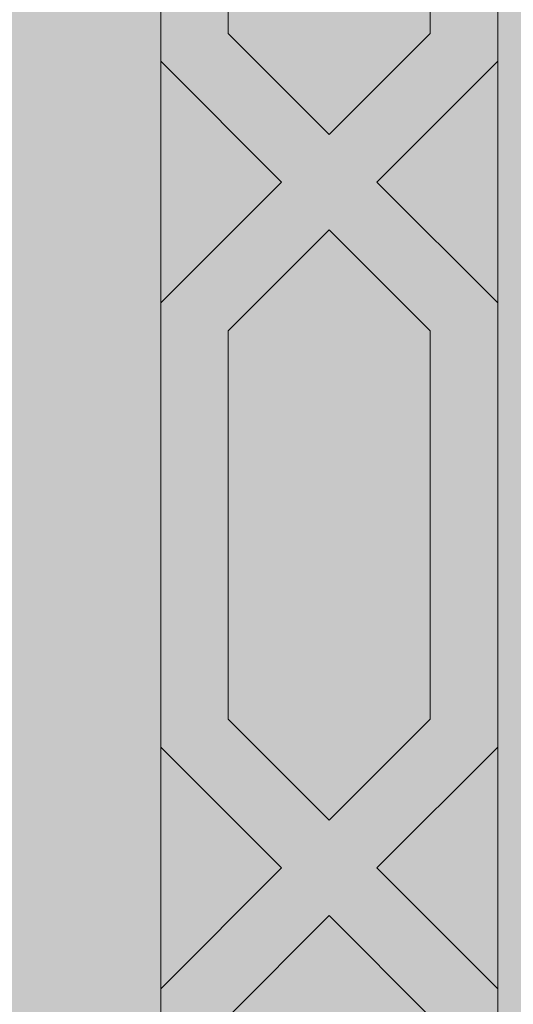
# Model space of a CAD drawing. Units: inches. Extents: x 844 to 2234, y 346 to 1084.
# Tile 86 of 93: x 2008.425 to 2010.294, y 706.497 to 710.224. Entities that reach past the tile are written whole.
import ezdxf

# ---------------------------------------------------------------- set-up
doc = ezdxf.new("R2010")
doc.units = ezdxf.units.IN
doc.header["$MEASUREMENT"] = 0
for name, color, linetype, lineweight in [('A-ANNO-DIMS', 2, 'Continuous', 18), ('furniture', 8, 'Continuous', 18), ('RA-AP-01$0$INT', 35, 'Continuous', 5)]:
    doc.layers.add(name, color=color, linetype=linetype, lineweight=lineweight)
doc.layers.add('RA-AP-01$0$FURN', color=3, linetype='Continuous')
doc.styles.get("Standard").update_dxf_attribs({"font": 'arial.ttf'})
doc.dimstyles.get("Standard").update_dxf_attribs({"dimtxt": 6, "dimasz": 3, "dimexe": 0.18, "dimexo": 0.0625, "dimgap": 0.09, "dimtad": 0, "dimtih": 1, "dimtoh": 1, "dimdec": 1, "dimzin": 0, "dimdsep": 46, "dimlunit": 3, "dimtxsty": 'Standard', "dimblk": 'ARCHTICK', "dimcen": 0.09, "dimadec": 0, "dimazin": 0, "dimtfac": 1, "dimtdec": 1, "dimtofl": 0, "dimtmove": 0, "dimatfit": 3, "dimfxl": 1, "dimtolj": 1, "dimtzin": 0, "dimarcsym": 0})

# ---------------------------------------------------------------- blocks, each defined once
blk = doc.blocks.new('A$C18D01794')
at = {"layer": 'RA-AP-01$0$INT'}
h = blk.add_hatch(color=256, dxfattribs=at)
h.paths.add_polyline_path([(4.355206456958071, -6.156712009588037), (4.355206456958071, -8.056712009588038), (5.455206456958072, -8.056712009588038), (5.455206456958072, -6.156712009588037)])
h.paths.add_polyline_path([(4.405206456958072, -8.006712009588039), (4.405206456958072, -6.206712009588038), (5.405206456958072, -6.206712009588038), (5.405206456958072, -8.006712009588039)], flags=16)
h = blk.add_hatch(color=256, dxfattribs=at)
h.paths.add_polyline_path([(4.505206456958071, -7.585498806127123), (4.46934859260189, -7.549640941759413), (4.505206456958071, -7.513783077414768), (4.505206456958071, -7.381963272220687), (4.469348592616735, -7.346105407867824), (4.505206456958071, -7.310247543514964), (4.505206456958071, -7.178427738324996), (4.469348592586679, -7.142569873965138), (4.505206456952245, -7.106712009588038), (4.476922185709333, -7.106712009588038), (4.455206456960671, -7.128427738343681), (4.433490728198047, -7.106712009588038), (4.405206456946033, -7.106712009588036), (4.441064321339216, -7.142569873969684), (4.40520645695807, -7.178427738362358), (4.405206456958072, -7.310247543472698), (4.441064321364728, -7.346105407867826), (4.40520645695807, -7.381963272262947), (4.40520645695807, -7.513783077378263), (4.441064321354429, -7.549640941786153), (4.405206456958072, -7.585498806170974), (4.405206456958072, -7.717318611286652), (4.441064321333084, -7.753176475673194), (4.405206456958072, -7.789034340036673), (4.405206456958072, -8.006712009588039), (4.644348592588106, -8.006712009588039), (4.680206456964639, -7.970854145211967), (4.716064321341165, -8.006712009588039), (4.869348592586113, -8.006712009588039), (4.905206456964143, -7.970854145210465), (4.941064321342174, -8.006712009588039), (5.094348592587118, -8.006712009588037), (5.130206456963649, -7.970854145211967), (5.166064321340178, -8.006712009588039), (5.405206456958072, -8.006712009588039), (5.405206456958072, -7.789034340024526), (5.369348592595202, -7.753176475673196), (5.40520645695807, -7.717318611298797), (5.40520645695807, -7.585498806158829), (5.369348592573859, -7.549640941786151), (5.40520645695807, -7.51378307739041), (5.40520645695807, -7.381963272250803), (5.36934859256356, -7.346105407867824), (5.405206456958072, -7.310247543484846), (5.405206456958072, -7.178427738350217), (5.369348592589068, -7.142569873969682), (5.405206456982249, -7.106712009588038), (5.376922185730244, -7.106712009588038), (5.355206456967613, -7.128427738343679), (5.333490728218955, -7.10671200958804), (5.305206456976043, -7.106712009588042), (5.341064321341609, -7.142569873965136), (5.305206456958072, -7.178427738337141), (5.305206456958072, -7.310247543502816), (5.34106432131155, -7.346105407867824), (5.305206456958072, -7.381963272232832), (5.30520645695807, -7.513783077402624), (5.341064321326395, -7.549640941759413), (5.305206456958072, -7.585498806139263), (5.305206456958072, -7.717318611299605), (5.341064321347738, -7.753176475677737), (5.305206456958072, -7.78903434007894), (5.30520645695807, -7.906712009588039), (5.166064321336834, -7.906712009588039), (5.130206456963647, -7.942569873961684), (5.094348592590464, -7.906712009588039), (4.941064321338827, -7.906712009588041), (4.905206456964145, -7.942569873963183), (4.869348592589459, -7.906712009588039), (4.716064321337822, -7.906712009588041), (4.680206456964641, -7.942569873961684), (4.644348592591453, -7.906712009588039), (4.505206456958071, -7.906712009588039), (4.505206456958071, -7.789034340066795), (4.469348592580545, -7.753176475677738), (4.505206456958071, -7.717318611311748)])
h.paths.add_polyline_path([(4.485206456974132, -7.709034340046354), (4.45520645695909, -7.739034340051736), (4.425206456974128, -7.709034340057131), (4.425206456993394, -7.593783077384998), (4.45520645699153, -7.563783077396511), (4.485206456993396, -7.593783077408017)], flags=16)
h.paths.add_polyline_path([(4.455206456954537, -7.767318611299197), (4.485206456958242, -7.797318611312542), (4.48520645695951, -7.912569873958716), (4.45520645695415, -7.942569873954422), (4.425206456957888, -7.912569873967813), (4.425206456957888, -7.797318611286197)], flags=16)
h.paths.add_polyline_path([(4.455206456964794, -7.535498806149051), (4.42520645696469, -7.5054988061393), (4.425206456983954, -7.390247543486406), (4.455206456990734, -7.360247543489279), (4.485206456983953, -7.39024754349214), (4.485206456964687, -7.505498806158811)], flags=16)
h.paths.add_polyline_path([(4.499348592588947, -7.926712009585049), (4.636064321340932, -7.926712009585049), (4.666064321342317, -7.956712009586821), (4.636064321343707, -7.986712009585048), (4.499348592575121, -7.986712009585048), (4.469348592591685, -7.956712009591957)], flags=16)
h.paths.add_polyline_path([(4.425206456957888, -7.940854145195974), (4.471064321332215, -7.986712009585049), (4.425206456957888, -7.986712009585049)], flags=16)
h.paths.add_polyline_path([(4.455206456990734, -7.331963272246367), (4.425206456989053, -7.301963272254337), (4.425206456969784, -7.186712009596224), (4.455206456965226, -7.156712009591144), (4.485206456969787, -7.186712009586051), (4.485206456989053, -7.301963272238404)], flags=16)
h.paths.add_polyline_path([(4.72434859258714, -7.926712009586255), (4.861064321340141, -7.926712009586248), (4.891064321340324, -7.956712009586823), (4.861064321340513, -7.986712009586252), (4.724348592586768, -7.986712009586252), (4.694348592586956, -7.956712009586821)], flags=16)
h.paths.add_polyline_path([(4.919348592587961, -7.956712009586821), (4.949348592588145, -7.92671200958625), (5.08606432134115, -7.926712009586253), (5.116064321341327, -7.956712009586823), (5.086064321341519, -7.986712009586252), (4.949348592587774, -7.986712009586252)], flags=16)
h.paths.add_polyline_path([(5.144348592585967, -7.956712009586823), (5.174348592587358, -7.926712009585049), (5.311064321339338, -7.926712009585049), (5.3410643213366, -7.956712009591957), (5.311064321353163, -7.986712009585048), (5.174348592584576, -7.986712009585048)], flags=16)
h.paths.add_polyline_path([(5.32520645693489, -7.593783077408021), (5.355206456936755, -7.563783077396511), (5.385206456934894, -7.593783077384998), (5.38520645695416, -7.709034340057128), (5.355206456969194, -7.739034340051736), (5.325206456954153, -7.709034340046352)], flags=16)
h.paths.add_polyline_path([(5.325206456970042, -7.797318611312542), (5.355206456973747, -7.767318611299197), (5.385206456970398, -7.7973186112862), (5.385206456970398, -7.912569873967816), (5.355206456974136, -7.942569873954422), (5.325206456968778, -7.912569873958716)], flags=16)
h.paths.add_polyline_path([(5.325206456963599, -7.505498806158811), (5.325206456944333, -7.39024754349214), (5.355206456937552, -7.360247543489279), (5.385206456944332, -7.39024754348641), (5.385206456963596, -7.505498806139303), (5.355206456963492, -7.53549880614905)], flags=16)
h.paths.add_polyline_path([(5.32520645693923, -7.301963272238403), (5.3252064569585, -7.186712009586051), (5.355206456963062, -7.156712009591142), (5.3852064569585, -7.186712009596224), (5.385206456939234, -7.301963272254338), (5.355206456937552, -7.331963272246369)], flags=16)
h.paths.add_polyline_path([(5.339348592596071, -7.986712009585048), (5.385206456970398, -7.940854145195972), (5.385206456970396, -7.986712009585048)], flags=16)
h = blk.add_hatch(color=256, dxfattribs=at)
h.paths.add_polyline_path([(4.469348592586677, -7.142569873965136), (4.505206456958073, -7.178427738324996), (4.505206456958071, -7.106712009582215)])
h.paths.add_polyline_path([(4.455206456960671, -7.128427738343681), (4.476922185709333, -7.106712009588038), (4.433490728198045, -7.106712009588038)])
h.paths.add_polyline_path([(4.405206456958073, -7.178427738362358), (4.441064321339218, -7.142569873969684), (4.40520645695807, -7.106712009600073)])
h.paths.add_polyline_path([(4.425206456989053, -7.301963272254335), (4.455206456990736, -7.331963272246371), (4.485206456989055, -7.301963272238399), (4.48520645696979, -7.186712009586054), (4.455206456965227, -7.15671200959114), (4.425206456969784, -7.186712009596224)])
h.paths.add_polyline_path([(4.505206456958073, -7.381963272220689), (4.505206456958071, -7.310247543514961), (4.469348592616738, -7.346105407867826)])
h.paths.add_polyline_path([(4.425206456964688, -7.5054988061393), (4.455206456964794, -7.535498806149051), (4.485206456964689, -7.505498806158811), (4.485206456983951, -7.390247543492138), (4.455206456990736, -7.360247543489277), (4.425206456983956, -7.39024754348641)])
h.paths.add_polyline_path([(4.425206456974126, -7.709034340057128), (4.455206456959092, -7.739034340051736), (4.485206456974132, -7.709034340046356), (4.485206456993396, -7.593783077408017), (4.45520645699153, -7.563783077396511), (4.425206456993394, -7.593783077384999)])
h.paths.add_polyline_path([(4.46934859260189, -7.549640941759415), (4.505206456958071, -7.585498806127123), (4.505206456958073, -7.513783077414766)])
h.paths.add_polyline_path([(4.405206456958073, -7.585498806170972), (4.441064321354427, -7.549640941786151), (4.405206456958072, -7.513783077378263)])
h.paths.add_polyline_path([(4.405206456958072, -7.789034340036673), (4.441064321333084, -7.753176475673194), (4.405206456958072, -7.71731861128665)])
h.paths.add_polyline_path([(4.469348592580547, -7.75317647567774), (4.505206456958071, -7.789034340066795), (4.505206456958071, -7.717318611311744)])
h.paths.add_polyline_path([(4.425206456957888, -7.912569873967814), (4.45520645695415, -7.942569873954422), (4.485206456959507, -7.912569873958718), (4.48520645695824, -7.797318611312542), (4.455206456954537, -7.767318611299197), (4.425206456957888, -7.797318611286202)])
h.paths.add_polyline_path([(4.425206456957888, -7.986712009585049), (4.471064321332215, -7.986712009585049), (4.425206456957888, -7.940854145195972)])
h.paths.add_polyline_path([(4.499348592575121, -7.986712009585048), (4.636064321343707, -7.986712009585049), (4.666064321342317, -7.956712009586823), (4.636064321340932, -7.926712009585049), (4.499348592588945, -7.926712009585049), (4.469348592591685, -7.95671200959196)])
h.paths.add_polyline_path([(4.680206456964641, -7.942569873961684), (4.716064321337824, -7.906712009588039), (4.644348592591454, -7.906712009588039)])
h.paths.add_polyline_path([(4.644348592588108, -8.006712009588039), (4.716064321341167, -8.006712009588039), (4.680206456964637, -7.970854145211964)])
h.paths.add_polyline_path([(4.724348592586768, -7.98671200958625), (4.861064321340514, -7.986712009586252), (4.891064321340324, -7.956712009586819), (4.861064321340141, -7.92671200958625), (4.724348592587134, -7.926712009586255), (4.694348592586957, -7.956712009586821)])
h.paths.add_polyline_path([(4.905206456964143, -7.942569873963183), (4.941064321338827, -7.906712009588039), (4.869348592589457, -7.906712009588037)])
h.paths.add_polyline_path([(4.869348592586113, -8.006712009588039), (4.941064321342172, -8.006712009588037), (4.905206456964145, -7.970854145210463)])
h.paths.add_polyline_path([(4.949348592587774, -7.986712009586252), (5.086064321341521, -7.986712009586252), (5.116064321341329, -7.956712009586823), (5.08606432134115, -7.926712009586253), (4.949348592588145, -7.92671200958625), (4.919348592587961, -7.956712009586819)])
h.paths.add_polyline_path([(5.130206456963645, -7.942569873961684), (5.166064321336834, -7.906712009588039), (5.094348592590464, -7.906712009588039)])
h.paths.add_polyline_path([(5.094348592587119, -8.006712009588039), (5.166064321340178, -8.006712009588039), (5.130206456963651, -7.970854145211967)])
h.paths.add_polyline_path([(5.174348592584578, -7.986712009585048), (5.311064321353163, -7.986712009585048), (5.341064321336602, -7.956712009591958), (5.31106432133934, -7.926712009585049), (5.174348592587352, -7.926712009585049), (5.144348592585969, -7.956712009586823)])
h.paths.add_polyline_path([(5.325206456968778, -7.912569873958718), (5.355206456974136, -7.942569873954422), (5.385206456970396, -7.912569873967814), (5.385206456970396, -7.797318611286199), (5.355206456973747, -7.767318611299197), (5.325206456970044, -7.797318611312544)])
h.paths.add_polyline_path([(5.339348592596073, -7.986712009585048), (5.385206456970396, -7.986712009585049), (5.385206456970398, -7.94085414519597)])
h.paths.add_polyline_path([(5.325206456954155, -7.709034340046354), (5.355206456969194, -7.739034340051734), (5.38520645695416, -7.709034340057128), (5.385206456934896, -7.593783077384999), (5.355206456936758, -7.563783077396513), (5.325206456934888, -7.593783077408019)])
h.paths.add_polyline_path([(5.305206456958072, -7.789034340078938), (5.341064321347739, -7.753176475677738), (5.305206456958072, -7.717318611299605)])
h.paths.add_polyline_path([(5.369348592595204, -7.753176475673194), (5.40520645695807, -7.789034340024526), (5.405206456958072, -7.717318611298798)])
h.paths.add_polyline_path([(5.405206456958072, -7.585498806158831), (5.405206456958072, -7.513783077390407), (5.369348592573857, -7.549640941786151)])
h.paths.add_polyline_path([(5.305206456958072, -7.585498806139266), (5.341064321326393, -7.549640941759413), (5.305206456958072, -7.513783077402626)])
h.paths.add_polyline_path([(5.325206456963599, -7.50549880615881), (5.355206456963494, -7.535498806149055), (5.385206456963598, -7.505498806139302), (5.385206456944334, -7.390247543486411), (5.355206456937552, -7.360247543489279), (5.325206456944333, -7.39024754349214)])
h.paths.add_polyline_path([(5.305206456958072, -7.38196327223283), (5.341064321311551, -7.346105407867824), (5.305206456958072, -7.31024754350282)])
h.paths.add_polyline_path([(5.325206456939231, -7.301963272238404), (5.355206456937552, -7.331963272246369), (5.385206456939235, -7.301963272254335), (5.385206456958502, -7.186712009596224), (5.355206456963061, -7.156712009591142), (5.3252064569585, -7.186712009586051)])
h.paths.add_polyline_path([(5.404581768715993, -7.381338584008926, -0.001217816984214), (5.405206456958072, -7.381112009582329), (5.405206456958072, -7.310247543484846), (5.369348592563558, -7.346105407867826)])
h.paths.add_polyline_path([(5.36934859258907, -7.142569873969684), (5.40520645695807, -7.178427738350215), (5.405206456958072, -7.106712009612218)])
h.paths.add_polyline_path([(5.355206456967613, -7.128427738343683), (5.376922185730239, -7.106712009588038), (5.333490728218953, -7.10671200958804)])
h.paths.add_polyline_path([(5.30520645695807, -7.178427738337139), (5.341064321341609, -7.142569873965134), (5.305206456958074, -7.10671200957007)])
blk.add_hatch(color=256, dxfattribs=at).paths.add_polyline_path([(4.505206456958071, -7.906712009588039), (5.305206456958072, -7.906712009588039), (5.305206456958072, -7.106712009588038), (5.255206456951893, -7.106712009588036), (5.25520645694868, -7.856712009570104), (4.555206456959269, -7.856712009588616), (4.555206456956052, -7.106712009588038), (4.505206456958073, -7.106712009588038)])
for p, q in [((4.425206456964688, -7.5054988061393), (4.455206456964796, -7.535498806149051)), ((4.485206456964687, -7.505498806158811), (4.455206456964796, -7.535498806149051)), ((4.405206456968717, -7.513783077388909), (4.441064321338788, -7.54964094177051)), ((4.505206456968717, -7.513783077404122), (4.469348592586251, -7.549640941775054)), ((4.405206456988469, -7.585498806140577), (4.441064321370071, -7.549640941770508)), ((4.505206456988468, -7.58549880615752), (4.469348592617532, -7.549640941775056)), ((4.425206456993394, -7.593783077384996), (4.45520645699153, -7.563783077396511)), ((4.485206456993396, -7.593783077408017), (4.45520645699153, -7.563783077396511)), ((4.425206456993394, -7.593783077384996), (4.425206456974128, -7.709034340057129)), ((4.485206456993396, -7.593783077408017), (4.485206456974132, -7.709034340046354)), ((4.425206456974128, -7.709034340057129), (4.455206456959092, -7.739034340051736)), ((4.485206456974132, -7.709034340046354), (4.455206456959092, -7.739034340051736)), ((4.405206456963013, -7.717318611291593), (4.441064321333084, -7.753176475673194)), ((4.505206456963013, -7.717318611306806), (4.469348592580547, -7.753176475677738)), ((4.441064321333084, -7.753176475673194), (4.405206456950156, -7.789034340044587)), ((4.469348592580547, -7.753176475677738), (4.505206456951941, -7.789034340060664)), ((4.455206456954537, -7.767318611299197), (4.425206456957888, -7.797318611286199)), ((4.455206456954537, -7.767318611299197), (4.485206456958242, -7.797318611312544)), ((4.425206456957888, -7.797318611286199), (4.425206456957888, -7.912569873967814)), ((4.485206456959509, -7.912569873958718), (4.485206456958242, -7.797318611312544))]:
    blk.add_line(p, q, dxfattribs=at)
for points in [[(5.405206456958072, -8.006712009588039), (4.405206456958072, -8.006712009588039), (4.405206456958072, -7.106712009588038)], [(5.305206456958072, -7.106712009588038), (5.305206456958072, -7.906712009588039), (4.505206456958071, -7.906712009588039), (4.505206456958071, -7.106712009588038)]]:
    blk.add_lwpolyline(points, dxfattribs=at)
blk = doc.blocks.new('A$C5D2F253E')
at = {"layer": 'RA-AP-01$0$FURN', "xscale": -0.7999999999883585, "yscale": 0.7999999999883585, "zscale": 0.8, "rotation": 90}
blk.add_blockref('A$C18D01794', (-5.687757199772477, 4.75791982714071), dxfattribs=at)
blk = doc.blocks.new('_ArchTick')
at = {"color": 0, "linetype": 'ByBlock', "const_width": 0.15}
blk.add_lwpolyline([(-0.5, -0.5), (0.5, 0.5)], dxfattribs=at)
blk = doc.blocks.new('*D121')
at = {"layer": 'A-ANNO-DIMS', "color": 0, "lineweight": -2, "transparency": 16777216}
for p, q in [((2030.271987351997, 734.262611118704), (2040.245275089302, 734.262611118704)), ((2040.065275089302, 734.262611118704), (2040.065275089302, 704.6043509484256)), ((2040.065275089302, 668.557359536674), (2040.065275089302, 698.2156197069523)), ((2030.271987351997, 668.557359536674), (2040.245275089302, 668.557359536674))]:
    blk.add_line(p, q, dxfattribs=at)
at = {"layer": 'Defpoints', "color": 0, "transparency": 16777216}
for p in [(2030.209487351997, 734.262611118704), (2040.065275089302, 734.262611118704), (2030.209487351997, 668.557359536674)]:
    blk.add_point(p, dxfattribs=at)
at = {"layer": 'A-ANNO-DIMS', "color": 0, "lineweight": -2, "transparency": 16777216, "xscale": 3, "yscale": 3, "zscale": 3}
for p, rotation in [((2040.065275089302, 734.262611118704), 90), ((2040.065275089302, 668.557359536674), 270)]:
    blk.add_blockref('_ArchTick', p, dxfattribs=dict(at, rotation=rotation))
at = {"layer": 'A-ANNO-DIMS', "color": 0, "transparency": 16777216, "insert": (2040.065275089302, 701.4099853276883), "char_height": 6, "attachment_point": 5}
blk.add_mtext('\\A1;LOUNGE SET 5\'-5 1/2" TYP.', dxfattribs=at)

msp = doc.modelspace()

# ---------------------------------------------------------------- block references
at = {"layer": 'furniture', "xscale": -15.94108302203742, "yscale": 15.94108302203742, "zscale": 15.94108302203742, "rotation": 270}
msp.add_blockref('A$C5D2F253E', (1990.567271852805, 701.4028671565849), dxfattribs=at)

# ---------------------------------------------------------------- dimensions: what is measured, and where the dimension line sits
at = {"layer": 'A-ANNO-DIMS'}
dim = msp.add_linear_dim(base=(2040.065275089302, 734.262611118704), p1=(2030.209487351996, 668.5573595366737), p2=(2030.209487351996, 734.2626111187037), angle=90, text='LOUNGE SET <> TYP.', dimstyle='Standard', override={"dimdec": 1, "dimlfac": 1, "dimrnd": 0, "dimzin": 1, "dimdsep": 46, "dimlunit": 4, "dimfrac": 2}, dxfattribs=at)
dim.commit()
dim.dimension.update_dxf_attribs({"geometry": '*D121', "text_midpoint": (2040.065275089302, 701.4099853276883)})

doc.saveas('drawing.dxf')
